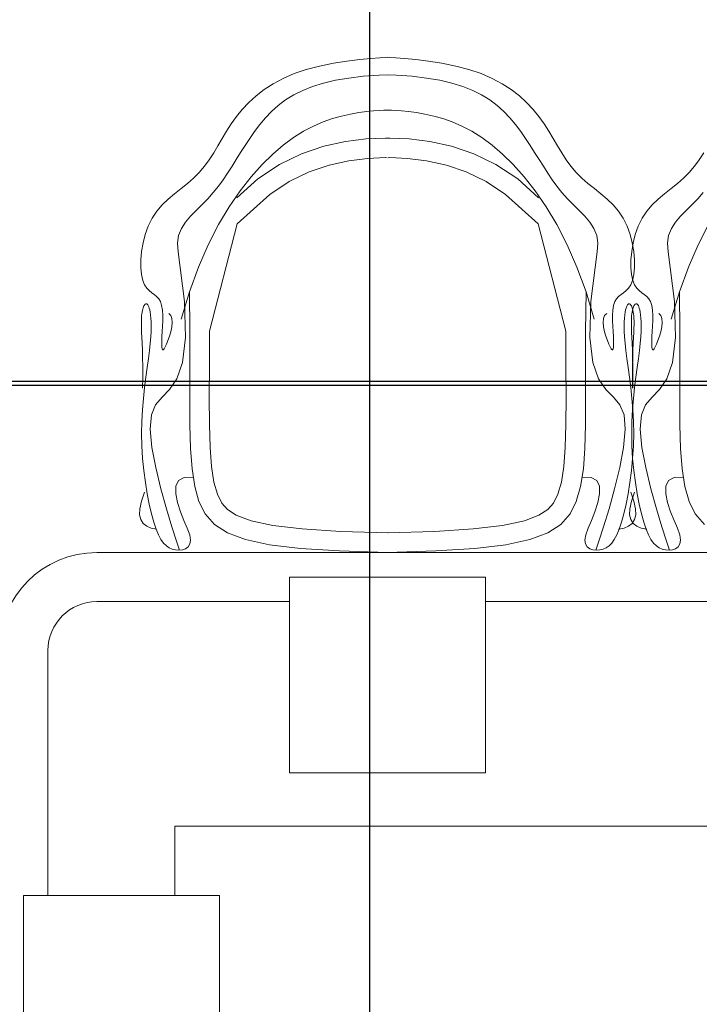
# Model space of a CAD drawing. Units: inches. Extents: x 1454 to 2136, y 626 to 1213.
# Tile 10 of 23: x 1592 to 1620, y 1101 to 1141. Entities that reach past the tile are written whole.
import ezdxf

# ---------------------------------------------------------------- set-up
doc = ezdxf.new("R2010")
doc.units = ezdxf.units.IN
doc.header["$MEASUREMENT"] = 0
for name, color, linetype, lineweight in [('A-ANNO-DIMS', 2, 'Continuous', 18), ('A-FURN-PATT', 252, 'Continuous', 13), ('conference', 41, 'Continuous', 18)]:
    doc.layers.add(name, color=color, linetype=linetype, lineweight=lineweight)
doc.styles.get("Standard").update_dxf_attribs({"font": 'arial.ttf'})
doc.dimstyles.get("Standard").update_dxf_attribs({"dimtxt": 4, "dimasz": 0.18, "dimexe": 0.18, "dimexo": 0.0625, "dimgap": 0.09, "dimtad": 0, "dimtih": 1, "dimtoh": 1, "dimdec": 0, "dimrnd": 6, "dimzin": 0, "dimdsep": 46, "dimlunit": 3, "dimtxsty": 'Standard', "dimcen": 0.09, "dimadec": 0, "dimazin": 0, "dimtfac": 1, "dimtdec": 0, "dimtofl": 0, "dimtmove": 0, "dimatfit": 3, "dimfxl": 1, "dimtolj": 1, "dimtzin": 0, "dimarcsym": 0})

# ---------------------------------------------------------------- blocks, each defined once
blk = doc.blocks.new('ОГ52_на12персон_стол2800х900')
for p, q in [((-1020.6, 783.7), (-1011.5, 784.5)), ((-1011.5, 784.5), (-1005.6, 784.9)), ((-1005.6, 784.9), (-1003.4, 785)), ((-1001.2, 784.9), (-1003.4, 785)), ((-995.2, 784.5), (-1001.2, 784.9)), ((-986.2, 783.7), (-995.2, 784.5)), ((-1086.4, 772.5), (-1072.8, 776)), ((-1072.8, 776), (-1058.8, 778.8)), ((-1058.8, 778.8), (-1044.9, 780.9)), ((-1044.9, 780.9), (-1031.9, 782.6)), ((-1031.9, 782.6), (-1020.6, 783.7)), ((-974.8, 782.6), (-986.2, 783.7)), ((-961.8, 780.9), (-974.8, 782.6)), ((-948, 778.8), (-961.8, 780.9)), ((-933.9, 776), (-948, 778.8)), ((-920.4, 772.5), (-933.9, 776)), ((-1110.1, 763.4), (-1098.8, 768.3)), ((-1098.8, 768.3), (-1086.4, 772.5)), ((-1043.1, 763.8), (-1028.3, 765.6)), ((-1028.3, 765.6), (-1012, 766.8)), ((-1012, 766.8), (-1003.4, 767.1)), ((-994.8, 766.8), (-1003.4, 767.1)), ((-978.4, 765.6), (-994.8, 766.8)), ((-963.6, 763.8), (-978.4, 765.6)), ((-907.9, 768.3), (-920.4, 772.5)), ((-896.6, 763.4), (-907.9, 768.3)), ((-1129.5, 752), (-1120.3, 758)), ((-1120.3, 758), (-1110.1, 763.4)), ((-1090.1, 751.2), (-1080, 755.2)), ((-1080, 755.2), (-1068.9, 758.7)), ((-1068.9, 758.7), (-1056.7, 761.5)), ((-1056.7, 761.5), (-1043.1, 763.8)), ((-950.1, 761.5), (-963.6, 763.8)), ((-937.8, 758.7), (-950.1, 761.5)), ((-926.7, 755.2), (-937.8, 758.7)), ((-916.6, 751.2), (-926.7, 755.2)), ((-886.5, 758), (-896.6, 763.4)), ((-877.3, 752), (-886.5, 758)), ((-1145.1, 738.8), (-1137.7, 745.6)), ((-1137.7, 745.6), (-1129.5, 752)), ((-1107.5, 741.4), (-1099.2, 746.6)), ((-1099.2, 746.6), (-1090.1, 751.2)), ((-907.5, 746.6), (-916.6, 751.2)), ((-899.2, 741.4), (-907.5, 746.6)), ((-869, 745.6), (-877.3, 752)), ((-861.6, 738.8), (-869, 745.6)), ((-1151.7, 731.7), (-1145.1, 738.8)), ((-1121.9, 729.6), (-1115, 735.7)), ((-1115, 735.7), (-1107.5, 741.4)), ((-891.7, 735.7), (-899.2, 741.4)), ((-884.9, 729.6), (-891.7, 735.7)), ((-855, 731.7), (-861.6, 738.8)), ((-1162.9, 716.9), (-1157.6, 724.4)), ((-1157.6, 724.4), (-1151.7, 731.7)), ((-1128.1, 723.1), (-1121.9, 729.6)), ((-1059.7, 722.3), (-1050.4, 724.9)), ((-1050.4, 724.9), (-1041.3, 727)), ((-1041.3, 727), (-1032.7, 728.5)), ((-1032.7, 728.5), (-1024.7, 729.6)), ((-1024.7, 729.6), (-1017.7, 730.4)), ((-1017.7, 730.4), (-1011.8, 730.8)), ((-1011.8, 730.8), (-1007.3, 731)), ((-1007.3, 731), (-1004.4, 731.1)), ((-1004.4, 731.1), (-1003.4, 731.1)), ((-1002.3, 731.1), (-1003.4, 731.1)), ((-999.4, 731), (-1002.3, 731.1)), ((-994.9, 730.8), (-999.4, 731)), ((-989.1, 730.4), (-994.9, 730.8)), ((-982, 729.6), (-989.1, 730.4)), ((-974.1, 728.5), (-982, 729.6)), ((-965.4, 727), (-974.1, 728.5)), ((-956.3, 724.9), (-965.4, 727)), ((-947, 722.3), (-956.3, 724.9)), ((-878.6, 723.1), (-884.9, 729.6)), ((-849.1, 724.4), (-855, 731.7)), ((-843.8, 716.9), (-849.1, 724.4)), ((-1167.7, 709.4), (-1162.9, 716.9)), ((-1139.2, 709.3), (-1133.9, 716.3)), ((-1133.9, 716.3), (-1128.1, 723.1)), ((-1089.1, 709.4), (-1079.1, 714.7)), ((-1079.1, 714.7), (-1069.3, 718.9)), ((-1069.3, 718.9), (-1059.7, 722.3)), ((-937.4, 718.9), (-947, 722.3)), ((-927.6, 714.7), (-937.4, 718.9)), ((-917.6, 709.4), (-927.6, 714.7)), ((-872.9, 716.3), (-878.6, 723.1)), ((-867.6, 709.3), (-872.9, 716.3)), ((-839, 709.4), (-843.8, 716.9)), ((-1172.2, 701.9), (-1167.7, 709.4)), ((-1144.1, 702.2), (-1139.2, 709.3)), ((-1099.4, 703), (-1089.1, 709.4)), ((-907.4, 703), (-917.6, 709.4)), ((-862.6, 702.2), (-867.6, 709.3)), ((-834.5, 701.9), (-839, 709.4)), ((-1180.9, 687.3), (-1176.6, 694.5)), ((-1176.6, 694.5), (-1172.2, 701.9)), ((-1153.4, 687.9), (-1148.8, 695)), ((-1148.8, 695), (-1144.1, 702.2)), ((-1120.6, 686.1), (-1109.9, 695.3)), ((-1109.9, 695.3), (-1099.4, 703)), ((-1091.2, 686.5), (-1068.6, 694.2)), ((-1068.6, 694.2), (-1046.5, 699)), ((-1046.5, 699), (-1025.4, 701.6)), ((-1025.4, 701.6), (-1005.7, 702.5)), ((-1005.7, 702.5), (-1003.4, 702.4)), ((-1001, 702.5), (-1003.4, 702.4)), ((-981.3, 701.6), (-1001, 702.5)), ((-960.2, 699), (-981.3, 701.6)), ((-938.1, 694.2), (-960.2, 699)), ((-915.6, 686.5), (-938.1, 694.2)), ((-896.9, 695.3), (-907.4, 703)), ((-886.2, 686.1), (-896.9, 695.3)), ((-857.9, 695), (-862.6, 702.2)), ((-853.4, 687.9), (-857.9, 695)), ((-830.2, 694.5), (-834.5, 701.9)), ((-825.8, 687.3), (-830.2, 694.5)), ((-1185.4, 680.3), (-1180.9, 687.3)), ((-1157.8, 680.7), (-1153.4, 687.9)), ((-1131.5, 675.4), (-1120.6, 686.1)), ((-1113.8, 675.6), (-1091.2, 686.5)), ((-893, 675.6), (-915.6, 686.5)), ((-875.2, 675.4), (-886.2, 686.1)), ((-848.9, 680.7), (-853.4, 687.9)), ((-821.3, 680.3), (-825.8, 687.3)), ((-685.4, 680.3), (-680.9, 687.3)), ((-1195.6, 667.5), (-1190.3, 673.7)), ((-1190.3, 673.7), (-1185.4, 680.3)), ((-1166.7, 666.7), (-1162.2, 673.7)), ((-1162.2, 673.7), (-1157.8, 680.7)), ((-1142.7, 663), (-1131.5, 675.4)), ((-1136, 660.8), (-1113.8, 675.6)), ((-1083.6, 668), (-1063.2, 674.9)), ((-1063.2, 674.9), (-1043.1, 679.3)), ((-1043.1, 679.3), (-1023.8, 681.7)), ((-1023.8, 681.7), (-1005.5, 682.5)), ((-1005.5, 682.5), (-1003.8, 682.4)), ((-1001.3, 682.5), (-1003, 682.4)), ((-983, 681.7), (-1001.3, 682.5)), ((-963.6, 679.3), (-983, 681.7)), ((-943.5, 674.9), (-963.6, 679.3)), ((-923.2, 668), (-943.5, 674.9)), ((-870.7, 660.8), (-893, 675.6)), ((-864, 663), (-875.2, 675.4)), ((-844.5, 673.7), (-848.9, 680.7)), ((-840.1, 666.7), (-844.5, 673.7)), ((-816.5, 673.7), (-821.3, 680.3)), ((-811.2, 667.5), (-816.5, 673.7)), ((-695.6, 667.5), (-690.3, 673.7)), ((-690.3, 673.7), (-685.4, 680.3)), ((-1201.4, 661.7), (-1195.6, 667.5)), ((-1171.3, 659.9), (-1166.7, 666.7)), ((-1103.8, 658.2), (-1083.6, 668)), ((-902.9, 658.2), (-923.2, 668)), ((-835.5, 659.9), (-840.1, 666.7)), ((-805.3, 661.7), (-811.2, 667.5)), ((-701.4, 661.7), (-695.6, 667.5)), ((-1214.2, 650.9), (-1207.7, 656.2)), ((-1207.7, 656.2), (-1201.4, 661.7)), ((-1176.1, 653.3), (-1171.3, 659.9)), ((-1157.3, 641.6), (-1136, 660.8)), ((-1154, 648.7), (-1142.7, 663)), ((-1123.7, 644.9), (-1103.8, 658.2)), ((-883, 644.9), (-902.9, 658.2)), ((-849.4, 641.6), (-870.7, 660.8)), ((-852.8, 648.7), (-864, 663)), ((-830.6, 653.3), (-835.5, 659.9)), ((-799, 656.2), (-805.3, 661.7)), ((-792.5, 650.9), (-799, 656.2)), ((-714.2, 650.9), (-707.7, 656.2)), ((-707.7, 656.2), (-701.4, 661.7)), ((-1227.3, 640.1), (-1220.8, 645.6)), ((-1220.8, 645.6), (-1214.2, 650.9)), ((-1186.8, 640.6), (-1181.3, 646.8)), ((-1181.3, 646.8), (-1176.1, 653.3)), ((-1165.2, 632.4), (-1154, 648.7)), ((-1157, 615), (-1123.7, 644.9)), ((-849.8, 615), (-883, 644.9)), ((-841.6, 632.4), (-852.8, 648.7)), ((-825.5, 646.8), (-830.6, 653.3)), ((-820, 640.6), (-825.5, 646.8)), ((-785.9, 645.6), (-792.5, 650.9)), ((-779.5, 640.1), (-785.9, 645.6)), ((-727.3, 640.1), (-720.8, 645.6)), ((-720.8, 645.6), (-714.2, 650.9)), ((-686.8, 640.6), (-681.3, 646.8)), ((-1238.9, 627.7), (-1233.4, 634.2)), ((-1233.4, 634.2), (-1227.3, 640.1)), ((-1198.7, 628.7), (-1192.7, 634.6)), ((-1192.7, 634.6), (-1186.8, 640.6)), ((-814.1, 634.6), (-820, 640.6)), ((-808, 628.7), (-814.1, 634.6)), ((-773.4, 634.2), (-779.5, 640.1)), ((-767.8, 627.7), (-773.4, 634.2)), ((-738.9, 627.7), (-733.4, 634.2)), ((-733.4, 634.2), (-727.3, 640.1)), ((-698.7, 628.7), (-692.7, 634.6)), ((-692.7, 634.6), (-686.8, 640.6)), ((-1243.7, 620.6), (-1238.9, 627.7)), ((-1204.5, 622.8), (-1198.7, 628.7)), ((-1176.1, 614.1), (-1165.2, 632.4)), ((-830.7, 614.1), (-841.6, 632.4)), ((-802.3, 622.8), (-808, 628.7)), ((-763, 620.6), (-767.8, 627.7)), ((-743.7, 620.6), (-738.9, 627.7)), ((-704.5, 622.8), (-698.7, 628.7)), ((-1247.7, 612.7), (-1243.7, 620.6)), ((-1213.8, 610.1), (-1209.6, 616.6)), ((-1209.6, 616.6), (-1204.5, 622.8)), ((-1186.6, 593.6), (-1176.1, 614.1)), ((-1157, 615), (-1185.3, 505.2)), ((-849.8, 615), (-821.5, 505.2)), ((-820.1, 593.6), (-830.7, 614.1)), ((-797.1, 616.6), (-802.3, 622.8)), ((-792.9, 610.1), (-797.1, 616.6)), ((-759.1, 612.7), (-763, 620.6)), ((-747.7, 612.7), (-743.7, 620.6)), ((-713.8, 610.1), (-709.6, 616.6)), ((-709.6, 616.6), (-704.5, 622.8)), ((-686.6, 593.6), (-676.1, 614.1)), ((-1253, 595.4), (-1250.7, 604.2)), ((-1250.7, 604.2), (-1247.7, 612.7)), ((-1216.7, 603), (-1213.8, 610.1)), ((-790, 603), (-792.9, 610.1)), ((-756, 604.2), (-759.1, 612.7)), ((-753.8, 595.4), (-756, 604.2)), ((-753, 595.4), (-750.7, 604.2)), ((-750.7, 604.2), (-747.7, 612.7)), ((-716.7, 603), (-713.8, 610.1)), ((-1254.4, 586.6), (-1253, 595.4)), ((-1217.9, 595.2), (-1216.7, 603)), ((-1217.1, 586.5), (-1217.9, 595.2)), ((-1196.5, 570.7), (-1186.6, 593.6)), ((-810.2, 570.7), (-820.1, 593.6)), ((-788.8, 595.2), (-790, 603)), ((-789.6, 586.5), (-788.8, 595.2)), ((-754.4, 586.6), (-753, 595.4)), ((-752.3, 586.6), (-753.8, 595.4)), ((-717.9, 595.2), (-716.7, 603)), ((-717.1, 586.5), (-717.9, 595.2)), ((-696.5, 570.7), (-686.6, 593.6)), ((-1255.1, 578.1), (-1254.4, 586.6)), ((-1217.1, 586.5), (-1210.8, 535.5)), ((-789.6, 586.5), (-796, 535.5)), ((-755.1, 578.1), (-754.4, 586.6)), ((-751.6, 578.1), (-752.3, 586.6)), ((-717.1, 586.5), (-710.8, 535.5)), ((-1255.1, 570.2), (-1255.1, 578.1)), ((-755.1, 570.2), (-755.1, 578.1)), ((-751.6, 570.2), (-751.6, 578.1)), ((-1254.5, 563.1), (-1255.1, 570.2)), ((-1253.2, 557.2), (-1254.5, 563.1)), ((-1205.7, 545.4), (-1196.5, 570.7)), ((-801, 545.4), (-810.2, 570.7)), ((-754.5, 563.1), (-755.1, 570.2)), ((-753.2, 557.2), (-754.5, 563.1)), ((-753.5, 557.2), (-752.3, 563.1)), ((-752.3, 563.1), (-751.6, 570.2)), ((-705.7, 545.4), (-696.5, 570.7)), ((-1251.4, 552.7), (-1253.2, 557.2)), ((-755.3, 552.7), (-753.5, 557.2)), ((-751.4, 552.7), (-753.2, 557.2)), ((-1249.2, 549.3), (-1251.4, 552.7)), ((-1246.7, 546.7), (-1249.2, 549.3)), ((-1244.1, 544.6), (-1246.7, 546.7)), ((-1241.5, 542.8), (-1244.1, 544.6)), ((-1214, 517.6), (-1205.7, 545.4)), ((-1205.7, 545.4), (-1205.3, 505.1)), ((-801, 545.4), (-801.5, 505.1)), ((-792.7, 517.6), (-801, 545.4)), ((-765.2, 542.8), (-762.6, 544.6)), ((-762.6, 544.6), (-760, 546.7)), ((-760, 546.7), (-757.5, 549.3)), ((-757.5, 549.3), (-755.3, 552.7)), ((-749.2, 549.3), (-751.4, 552.7)), ((-746.7, 546.7), (-749.2, 549.3)), ((-744.1, 544.6), (-746.7, 546.7)), ((-741.5, 542.8), (-744.1, 544.6)), ((-714, 517.6), (-705.7, 545.4)), ((-705.7, 545.4), (-705.3, 505.1)), ((-1250.7, 533), (-1251.2, 532.5)), ((-1250.2, 533.2), (-1250.7, 533)), ((-1249.7, 533.3), (-1250.2, 533.2)), ((-1249.2, 533.2), (-1249.7, 533.3)), ((-1248.7, 532.9), (-1249.2, 533.2)), ((-1248.1, 532.3), (-1248.7, 532.9)), ((-1239.1, 540.8), (-1241.5, 542.8)), ((-1236.9, 538.5), (-1239.1, 540.8)), ((-1235.2, 535.5), (-1236.9, 538.5)), ((-1234, 531.5), (-1235.2, 535.5)), ((-1210.8, 535.5), (-1209.7, 498.8)), ((-796, 535.5), (-797, 498.8)), ((-772.8, 531.5), (-771.6, 535.5)), ((-771.6, 535.5), (-769.8, 538.5)), ((-769.8, 538.5), (-767.7, 540.8)), ((-767.7, 540.8), (-765.2, 542.8)), ((-758.6, 532.3), (-758.1, 532.9)), ((-758.1, 532.9), (-757.6, 533.2)), ((-757.6, 533.2), (-757, 533.3)), ((-757, 533.3), (-756.5, 533.2)), ((-756.5, 533.2), (-756, 533)), ((-756, 533), (-755.6, 532.5)), ((-750.7, 533), (-751.2, 532.5)), ((-750.2, 533.2), (-750.7, 533)), ((-749.7, 533.3), (-750.2, 533.2)), ((-749.2, 533.2), (-749.7, 533.3)), ((-748.7, 532.9), (-749.2, 533.2)), ((-748.1, 532.3), (-748.7, 532.9)), ((-739.1, 540.8), (-741.5, 542.8)), ((-736.9, 538.5), (-739.1, 540.8)), ((-735.2, 535.5), (-736.9, 538.5)), ((-734, 531.5), (-735.2, 535.5)), ((-710.8, 535.5), (-709.7, 498.8)), ((-1254.2, 523.1), (-1254.5, 521)), ((-1254, 524.9), (-1254.2, 523.1)), ((-1253.6, 526.5), (-1254, 524.9)), ((-1253.3, 527.9), (-1253.6, 526.5)), ((-1252.9, 529.1), (-1253.3, 527.9)), ((-1252.5, 530.2), (-1252.9, 529.1)), ((-1252.1, 531.1), (-1252.5, 530.2)), ((-1251.6, 531.9), (-1252.1, 531.1)), ((-1251.2, 532.5), (-1251.6, 531.9)), ((-1247.6, 531.5), (-1248.1, 532.3)), ((-1247.1, 530.3), (-1247.6, 531.5)), ((-1246.6, 528.8), (-1247.1, 530.3)), ((-1246.2, 527), (-1246.6, 528.8)), ((-1245.7, 524.7), (-1246.2, 527)), ((-1245.3, 521.9), (-1245.7, 524.7)), ((-1233.3, 526.8), (-1234, 531.5)), ((-1232.9, 521.5), (-1233.3, 526.8)), ((-1226.8, 523.4), (-1224.6, 521.4)), ((-779.9, 523.4), (-782.1, 521.4)), ((-773.8, 521.5), (-773.5, 526.8)), ((-773.5, 526.8), (-772.8, 531.5)), ((-761.4, 521.9), (-761, 524.7)), ((-761, 524.7), (-760.6, 527)), ((-760.6, 527), (-760.1, 528.8)), ((-760.1, 528.8), (-759.6, 530.3)), ((-759.6, 530.3), (-759.1, 531.5)), ((-759.1, 531.5), (-758.6, 532.3)), ((-755.6, 532.5), (-755.1, 531.9)), ((-755.1, 531.9), (-754.7, 531.1)), ((-754.7, 531.1), (-754.2, 530.2)), ((-754.2, 523.1), (-754.5, 521)), ((-754.2, 530.2), (-753.8, 529.1)), ((-754, 524.9), (-754.2, 523.1)), ((-753.6, 526.5), (-754, 524.9)), ((-753.8, 529.1), (-753.5, 527.9)), ((-753.3, 527.9), (-753.6, 526.5)), ((-753.5, 527.9), (-753.1, 526.5)), ((-752.9, 529.1), (-753.3, 527.9)), ((-753.1, 526.5), (-752.8, 524.9)), ((-752.5, 530.2), (-752.9, 529.1)), ((-752.8, 524.9), (-752.5, 523.1)), ((-752.1, 531.1), (-752.5, 530.2)), ((-752.5, 523.1), (-752.3, 521)), ((-751.6, 531.9), (-752.1, 531.1)), ((-751.2, 532.5), (-751.6, 531.9)), ((-747.6, 531.5), (-748.1, 532.3)), ((-747.1, 530.3), (-747.6, 531.5)), ((-746.6, 528.8), (-747.1, 530.3)), ((-746.2, 527), (-746.6, 528.8)), ((-745.7, 524.7), (-746.2, 527)), ((-745.3, 521.9), (-745.7, 524.7)), ((-733.3, 526.8), (-734, 531.5)), ((-732.9, 521.5), (-733.3, 526.8)), ((-726.8, 523.4), (-724.6, 521.4)), ((-1254.6, 518.5), (-1254.7, 515.7)), ((-1254.7, 515.7), (-1254.7, 512.3)), ((-1254.5, 521), (-1254.6, 518.5)), ((-1245, 518.7), (-1245.3, 521.9)), ((-1244.8, 514.9), (-1245, 518.7)), ((-1244.7, 510.5), (-1244.8, 514.9)), ((-1233.1, 510.3), (-1232.9, 516)), ((-1232.9, 516), (-1232.9, 521.5)), ((-1224.6, 521.4), (-1223.5, 518.2)), ((-1223.3, 514.2), (-1223.7, 509.6)), ((-1223.5, 518.2), (-1223.3, 514.2)), ((-783.2, 518.2), (-783.5, 514.2)), ((-783.5, 514.2), (-783, 509.6)), ((-782.1, 521.4), (-783.2, 518.2)), ((-773.8, 516), (-773.8, 521.5)), ((-773.6, 510.3), (-773.8, 516)), ((-762, 510.5), (-761.9, 514.9)), ((-761.9, 514.9), (-761.7, 518.7)), ((-761.7, 518.7), (-761.4, 521.9)), ((-754.6, 518.5), (-754.7, 515.7)), ((-754.7, 515.7), (-754.7, 512.3)), ((-754.5, 521), (-754.6, 518.5)), ((-752.3, 521), (-752.1, 518.5)), ((-752.1, 518.5), (-752, 515.7)), ((-752, 515.7), (-752, 512.3)), ((-745, 518.7), (-745.3, 521.9)), ((-744.8, 514.9), (-745, 518.7)), ((-744.7, 510.5), (-744.8, 514.9)), ((-733.1, 510.3), (-732.9, 516)), ((-732.9, 516), (-732.9, 521.5)), ((-724.6, 521.4), (-723.5, 518.2)), ((-723.3, 514.2), (-723.7, 509.6)), ((-723.5, 518.2), (-723.3, 514.2)), ((-1254.7, 512.3), (-1254.6, 508.5)), ((-1254.6, 508.5), (-1254.5, 504)), ((-1254.5, 504), (-1254.2, 498.9)), ((-1245.1, 499.6), (-1244.8, 505.4)), ((-1244.8, 505.4), (-1244.7, 510.5)), ((-1233.7, 499.8), (-1233.4, 504.9)), ((-1233.4, 504.9), (-1233.1, 510.3)), ((-1224.7, 504.8), (-1226.1, 500.1)), ((-1223.7, 509.6), (-1224.7, 504.8)), ((-1205.3, 505.1), (-1205.3, 469.2)), ((-1185.3, 505.2), (-1185.3, 469.2)), ((-821.5, 505.2), (-821.5, 469.2)), ((-801.5, 505.1), (-801.5, 469.2)), ((-783, 509.6), (-782, 504.8)), ((-782, 504.8), (-780.7, 500.1)), ((-773.4, 504.9), (-773.6, 510.3)), ((-773.1, 499.8), (-773.4, 504.9)), ((-762, 505.4), (-762, 510.5)), ((-761.7, 499.6), (-762, 505.4)), ((-754.7, 512.3), (-754.6, 508.5)), ((-754.6, 508.5), (-754.5, 504)), ((-754.5, 504), (-754.2, 498.9)), ((-752.3, 504), (-752.5, 498.9)), ((-752.1, 508.5), (-752.3, 504)), ((-752, 512.3), (-752.1, 508.5)), ((-745.1, 499.6), (-744.8, 505.4)), ((-744.8, 505.4), (-744.7, 510.5)), ((-733.7, 499.8), (-733.4, 504.9)), ((-733.4, 504.9), (-733.1, 510.3)), ((-724.7, 504.8), (-726.1, 500.1)), ((-723.7, 509.6), (-724.7, 504.8)), ((-705.3, 505.1), (-705.3, 469.2)), ((-1254.2, 498.9), (-1253.9, 493)), ((-1253.9, 493), (-1253.7, 486.1)), ((-1246.4, 485.6), (-1245.6, 493.1)), ((-1245.6, 493.1), (-1245.1, 499.6)), ((-1233.9, 495.4), (-1233.7, 499.8)), ((-1233.9, 491.8), (-1233.9, 495.4)), ((-1227.6, 495.7), (-1229, 492)), ((-1226.1, 500.1), (-1227.6, 495.7)), ((-1209.7, 498.8), (-1212.8, 473.4)), ((-797, 498.8), (-794, 473.4)), ((-780.7, 500.1), (-779.2, 495.7)), ((-779.2, 495.7), (-777.7, 492)), ((-772.9, 495.4), (-773.1, 499.8)), ((-772.8, 491.8), (-772.9, 495.4)), ((-761.2, 493.1), (-761.7, 499.6)), ((-760.4, 485.6), (-761.2, 493.1)), ((-754.2, 498.9), (-753.9, 493)), ((-753.9, 493), (-753.7, 486.1)), ((-752.8, 493), (-753.1, 486.1)), ((-752.5, 498.9), (-752.8, 493)), ((-746.4, 485.6), (-745.6, 493.1)), ((-745.6, 493.1), (-745.1, 499.6)), ((-733.9, 495.4), (-733.7, 499.8)), ((-733.9, 491.8), (-733.9, 495.4)), ((-727.6, 495.7), (-729, 492)), ((-726.1, 500.1), (-727.6, 495.7)), ((-709.7, 498.8), (-712.8, 473.4)), ((-1253.7, 486.1), (-1253.4, 478.2)), ((-1247.4, 477.3), (-1246.4, 485.6)), ((-1233.8, 489.1), (-1233.9, 491.8)), ((-1233.5, 487.3), (-1233.8, 489.1)), ((-1233, 486.4), (-1233.5, 487.3)), ((-1232.3, 486.4), (-1233, 486.4)), ((-1231.4, 487.3), (-1232.3, 486.4)), ((-1230.3, 489.2), (-1231.4, 487.3)), ((-1229, 492), (-1230.3, 489.2)), ((-777.7, 492), (-776.4, 489.2)), ((-776.4, 489.2), (-775.3, 487.3)), ((-775.3, 487.3), (-774.4, 486.4)), ((-774.4, 486.4), (-773.8, 486.4)), ((-773.8, 486.4), (-773.3, 487.3)), ((-773.3, 487.3), (-772.9, 489.1)), ((-772.9, 489.1), (-772.8, 491.8)), ((-759.3, 477.3), (-760.4, 485.6)), ((-753.7, 486.1), (-753.4, 478.2)), ((-753.1, 486.1), (-753.3, 478.2)), ((-747.4, 477.3), (-746.4, 485.6)), ((-733.8, 489.1), (-733.9, 491.8)), ((-733.5, 487.3), (-733.8, 489.1)), ((-733, 486.4), (-733.5, 487.3)), ((-732.3, 486.4), (-733, 486.4)), ((-731.4, 487.3), (-732.3, 486.4)), ((-730.3, 489.2), (-731.4, 487.3)), ((-729, 492), (-730.3, 489.2)), ((-1253.4, 478.2), (-1253.3, 469.2)), ((-1248.7, 468.2), (-1247.4, 477.3)), ((-1212.8, 473.4), (-1218.6, 456.6)), ((-794, 473.4), (-788.1, 456.6)), ((-758, 468.2), (-759.3, 477.3)), ((-753.3, 478.2), (-753.4, 469.2)), ((-753.4, 478.2), (-753.3, 469.2)), ((-748.7, 468.2), (-747.4, 477.3)), ((-712.8, 473.4), (-718.6, 456.6)), ((-1253.3, 469.2), (-1253.3, 458.8)), ((-1250, 458.3), (-1248.7, 468.2)), ((-1205.3, 469.2), (-1205.4, 437.5)), ((-1185.3, 469.2), (-1185.4, 437.6)), ((-821.5, 469.2), (-821.4, 437.6)), ((-801.5, 469.2), (-801.4, 437.5)), ((-756.7, 458.3), (-758, 468.2)), ((-753.4, 469.2), (-753.5, 458.8)), ((-753.3, 469.2), (-753.3, 458.8)), ((-750, 458.3), (-748.7, 468.2)), ((-705.3, 469.2), (-705.4, 437.5)), ((-1253.3, 458.8), (-1253.4, 447.1)), ((-1251.4, 447.8), (-1250, 458.3)), ((-1218.6, 456.6), (-1226, 445.7)), ((-788.1, 456.6), (-780.7, 445.7)), ((-755.4, 447.8), (-756.7, 458.3)), ((-753.5, 458.8), (-753.3, 447.1)), ((-753.3, 458.8), (-753.4, 447.1)), ((-751.4, 447.8), (-750, 458.3)), ((-718.6, 456.6), (-726, 445.7)), ((-1252.6, 436.7), (-1251.4, 447.8)), ((-1226, 445.7), (-1233.6, 437.8)), ((-780.7, 445.7), (-773.1, 437.8)), ((-754.1, 436.7), (-755.4, 447.8)), ((-752.6, 436.7), (-751.4, 447.8)), ((-726, 445.7), (-733.6, 437.8)), ((-1253.6, 425.1), (-1252.6, 436.7)), ((-1233.6, 437.8), (-1240.2, 430.2)), ((-1205.4, 437.5), (-1205.3, 409.8)), ((-1185.4, 437.6), (-1185.3, 410.1)), ((-821.4, 437.6), (-821.5, 410.1)), ((-801.4, 437.5), (-801.5, 409.8)), ((-773.1, 437.8), (-766.5, 430.2)), ((-753.1, 425.1), (-754.1, 436.7)), ((-753.6, 425.1), (-752.6, 436.7)), ((-733.6, 437.8), (-740.2, 430.2)), ((-705.4, 437.5), (-705.3, 409.8)), ((-1254.2, 413.1), (-1253.6, 425.1)), ((-1240.2, 430.2), (-1244.5, 420)), ((-766.5, 430.2), (-762.2, 420)), ((-754.2, 413.1), (-753.6, 425.1)), ((-752.5, 413.1), (-753.1, 425.1)), ((-740.2, 430.2), (-744.5, 420)), ((-1254.4, 400.7), (-1254.2, 413.1)), ((-1244.5, 420), (-1245.6, 405.3)), ((-762.2, 420), (-761.1, 405.3)), ((-754.4, 400.7), (-754.2, 413.1)), ((-752.3, 400.7), (-752.5, 413.1)), ((-744.5, 420), (-745.6, 405.3)), ((-1245.6, 405.3), (-1243.9, 386.7)), ((-1205.3, 409.8), (-1204.6, 385.6)), ((-1185.3, 410.1), (-1184.6, 386.6)), ((-821.5, 410.1), (-822.1, 386.6)), ((-801.5, 409.8), (-802.2, 385.6)), ((-761.1, 405.3), (-762.8, 386.7)), ((-745.6, 405.3), (-743.9, 386.7)), ((-705.3, 409.8), (-704.6, 385.6)), ((-1254.1, 388.2), (-1254.4, 400.7)), ((-754.1, 388.2), (-754.4, 400.7)), ((-752.6, 388.2), (-752.3, 400.7)), ((-1253.4, 375.5), (-1254.1, 388.2)), ((-1243.9, 386.7), (-1240.1, 366)), ((-1204.6, 385.6), (-1203, 364.7)), ((-1184.6, 386.6), (-1183.1, 367)), ((-822.1, 386.6), (-823.6, 367)), ((-802.2, 385.6), (-803.7, 364.7)), ((-762.8, 386.7), (-766.6, 366)), ((-753.4, 375.5), (-754.1, 388.2)), ((-753.4, 375.5), (-752.6, 388.2)), ((-743.9, 386.7), (-740.1, 366)), ((-704.6, 385.6), (-703, 364.7)), ((-1252.1, 363), (-1253.4, 375.5)), ((-754.6, 363), (-753.4, 375.5)), ((-752.1, 363), (-753.4, 375.5)), ((-1250.6, 350.9), (-1252.1, 363)), ((-1240.1, 366), (-1235, 344.5)), ((-1203, 364.7), (-1200.2, 346.8)), ((-1183.1, 367), (-1180.6, 351.1)), ((-823.6, 367), (-826.1, 351.1)), ((-803.7, 364.7), (-806.5, 346.8)), ((-766.6, 366), (-771.8, 344.5)), ((-756.2, 350.9), (-754.6, 363)), ((-750.6, 350.9), (-752.1, 363)), ((-740.1, 366), (-735, 344.5)), ((-703, 364.7), (-700.2, 346.8)), ((-1219.4, 347.1), (-1216.8, 353)), ((-1216.8, 353), (-1211.1, 356.1)), ((-1211.1, 356.1), (-1201.6, 355.7)), ((-795.6, 356.1), (-805.1, 355.7)), ((-789.9, 353), (-795.6, 356.1)), ((-787.3, 347.1), (-789.9, 353)), ((-719.4, 347.1), (-716.8, 353)), ((-716.8, 353), (-711.1, 356.1)), ((-711.1, 356.1), (-701.6, 355.7)), ((-1248.7, 339.4), (-1250.6, 350.9)), ((-1235, 344.5), (-1229.2, 323.8)), ((-1219.5, 339.3), (-1219.4, 347.1)), ((-1200.2, 346.8), (-1195.9, 331.5)), ((-1180.6, 351.1), (-1177.1, 338.8)), ((-826.1, 351.1), (-829.6, 338.8)), ((-806.5, 346.8), (-810.9, 331.5)), ((-787.3, 339.3), (-787.3, 347.1)), ((-771.8, 344.5), (-777.5, 323.8)), ((-758, 339.4), (-756.2, 350.9)), ((-748.7, 339.4), (-750.6, 350.9)), ((-735, 344.5), (-729.2, 323.8)), ((-719.5, 339.3), (-719.4, 347.1)), ((-700.2, 346.8), (-695.9, 331.5)), ((-1254.7, 331.8), (-1256.3, 324.1)), ((-1251.4, 341), (-1254.7, 331.8)), ((-1246.6, 328.7), (-1248.7, 339.4)), ((-1217.7, 330.3), (-1219.5, 339.3)), ((-1177.1, 338.8), (-1172.7, 329.9)), ((-829.6, 338.8), (-834, 329.9)), ((-789.1, 330.3), (-787.3, 339.3)), ((-760.1, 328.7), (-758, 339.4)), ((-754.7, 331.8), (-756.3, 324.1)), ((-755.4, 341), (-752.1, 331.8)), ((-751.4, 341), (-754.7, 331.8)), ((-752.1, 331.8), (-750.4, 324.1)), ((-746.6, 328.7), (-748.7, 339.4)), ((-717.7, 330.3), (-719.5, 339.3)), ((-1256.3, 324.1), (-1256.5, 317.8)), ((-1244.4, 318.9), (-1246.6, 328.7)), ((-1229.2, 323.8), (-1223.6, 305.4)), ((-1214.7, 321), (-1217.7, 330.3)), ((-1195.9, 331.5), (-1189.5, 318.7)), ((-1172.7, 329.9), (-1166.9, 323.3)), ((-1166.9, 323.3), (-1157.8, 317.4)), ((-839.8, 323.3), (-849, 317.4)), ((-834, 329.9), (-839.8, 323.3)), ((-810.9, 331.5), (-817.3, 318.7)), ((-792, 321), (-789.1, 330.3)), ((-777.5, 323.8), (-783.1, 305.4)), ((-762.3, 318.9), (-760.1, 328.7)), ((-756.3, 324.1), (-756.5, 317.8)), ((-750.4, 324.1), (-750.2, 317.8)), ((-744.4, 318.9), (-746.6, 328.7)), ((-729.2, 323.8), (-723.6, 305.4)), ((-714.7, 321), (-717.7, 330.3)), ((-695.9, 331.5), (-689.5, 318.7)), ((-1256.5, 317.8), (-1255.3, 312.9)), ((-1255.3, 312.9), (-1252.8, 309)), ((-1242.1, 310.4), (-1244.4, 318.9)), ((-1211.2, 312), (-1214.7, 321)), ((-1207.8, 304.2), (-1211.2, 312)), ((-1189.5, 318.7), (-1180.2, 308)), ((-1157.8, 317.4), (-1142.8, 311.8)), ((-1142.8, 311.8), (-1120.7, 307)), ((-863.9, 311.8), (-886.1, 307)), ((-849, 317.4), (-863.9, 311.8)), ((-817.3, 318.7), (-826.6, 308)), ((-798.9, 304.2), (-795.5, 312)), ((-795.5, 312), (-792, 321)), ((-764.7, 310.4), (-762.3, 318.9)), ((-756.5, 317.8), (-755.3, 312.9)), ((-755.3, 312.9), (-752.8, 309)), ((-751.5, 312.9), (-754, 309)), ((-750.2, 317.8), (-751.5, 312.9)), ((-742.1, 310.4), (-744.4, 318.9)), ((-711.2, 312), (-714.7, 321)), ((-707.8, 304.2), (-711.2, 312)), ((-689.5, 318.7), (-680.2, 308)), ((-1252.8, 309), (-1249.2, 306.2)), ((-1249.2, 306.2), (-1244.6, 304.3)), ((-1244.6, 304.3), (-1239.1, 303.1)), ((-1239.7, 303.2), (-1242.1, 310.4)), ((-1237.2, 297.3), (-1239.7, 303.2)), ((-1223.6, 305.4), (-1218.9, 291)), ((-1207.8, 304.2), (-1205.4, 297.4)), ((-1180.2, 308), (-1166.8, 299.4)), ((-1120.7, 307), (-1090.5, 303.4)), ((-1090.5, 303.4), (-1051.5, 300.9)), ((-916.3, 303.4), (-955.2, 300.9)), ((-886.1, 307), (-916.3, 303.4)), ((-826.6, 308), (-839.9, 299.4)), ((-798.9, 304.2), (-801.3, 297.4)), ((-783.1, 305.4), (-787.8, 291)), ((-769.5, 297.3), (-767.1, 303.2)), ((-762.2, 304.3), (-767.7, 303.1)), ((-767.1, 303.2), (-764.7, 310.4)), ((-757.6, 306.2), (-762.2, 304.3)), ((-754, 309), (-757.6, 306.2)), ((-752.8, 309), (-749.2, 306.2)), ((-749.2, 306.2), (-744.6, 304.3)), ((-744.6, 304.3), (-739.1, 303.1)), ((-739.7, 303.2), (-742.1, 310.4)), ((-737.2, 297.3), (-739.7, 303.2)), ((-723.6, 305.4), (-718.9, 291)), ((-707.8, 304.2), (-705.4, 297.4)), ((-1234.7, 292.5), (-1237.2, 297.3)), ((-1232, 288.8), (-1234.7, 292.5)), ((-1205.4, 297.4), (-1204.6, 292.1)), ((-1204.6, 292.1), (-1205.3, 288.1)), ((-1166.8, 299.4), (-1148.5, 292.5)), ((-1148.5, 292.5), (-1124, 287.3)), ((-1051.5, 300.9), (-1002.7, 299.3)), ((-955.2, 300.9), (-1004, 299.3)), ((-858.3, 292.5), (-882.8, 287.3)), ((-839.9, 299.4), (-858.3, 292.5)), ((-801.3, 297.4), (-802.1, 292.1)), ((-802.1, 292.1), (-801.5, 288.1)), ((-774.7, 288.8), (-772.1, 292.5)), ((-772.1, 292.5), (-769.5, 297.3)), ((-734.7, 292.5), (-737.2, 297.3)), ((-732, 288.8), (-734.7, 292.5)), ((-705.4, 297.4), (-704.6, 292.1)), ((-704.6, 292.1), (-705.3, 288.1)), ((-1229.2, 286.1), (-1232, 288.8)), ((-1226.3, 284.1), (-1229.2, 286.1)), ((-1223.2, 282.8), (-1226.3, 284.1)), ((-1219.8, 282.1), (-1223.2, 282.8)), ((-1216.3, 281.8), (-1219.8, 282.1)), ((-1218.9, 291), (-1215.9, 281.9)), ((-1212.8, 282.2), (-1216.3, 281.8)), ((-1209.6, 283.2), (-1212.8, 282.2)), ((-1207, 285.1), (-1209.6, 283.2)), ((-1205.3, 288.1), (-1207, 285.1)), ((-1124, 287.3), (-1092.3, 283.5)), ((-1092.3, 283.5), (-1052.5, 280.9)), ((-914.4, 283.5), (-954.3, 280.9)), ((-882.8, 287.3), (-914.4, 283.5)), ((-801.5, 288.1), (-799.7, 285.1)), ((-799.7, 285.1), (-797.1, 283.2)), ((-797.1, 283.2), (-793.9, 282.2)), ((-793.9, 282.2), (-790.4, 281.8)), ((-787.8, 291), (-790.9, 281.9)), ((-790.4, 281.8), (-786.9, 282.1)), ((-786.9, 282.1), (-783.6, 282.8)), ((-783.6, 282.8), (-780.4, 284.1)), ((-780.4, 284.1), (-777.5, 286.1)), ((-777.5, 286.1), (-774.7, 288.8)), ((-729.2, 286.1), (-732, 288.8)), ((-726.3, 284.1), (-729.2, 286.1)), ((-723.2, 282.8), (-726.3, 284.1)), ((-719.8, 282.1), (-723.2, 282.8)), ((-716.3, 281.8), (-719.8, 282.1)), ((-718.9, 291), (-715.9, 281.9)), ((-712.8, 282.2), (-716.3, 281.8)), ((-709.6, 283.2), (-712.8, 282.2)), ((-707, 285.1), (-709.6, 283.2)), ((-705.3, 288.1), (-707, 285.1)), ((-1300, 279.3), (1300, 279.3)), ((-1052.5, 280.9), (-1003.4, 279.3)), ((-954.3, 280.9), (-1003.4, 279.3)), ((-1103.4, 54.3), (-1103.4, 254.3)), ((-1103.4, 254.3), (-903.4, 254.3)), ((-903.4, 254.3), (-903.4, 54.3)), ((-1103.4, 229.3), (-1300, 229.3)), ((-603.4, 229.3), (-903.4, 229.3)), ((-1350, 179.3), (-1350, -70.7)), ((-903.4, 54.3), (-1103.4, 54.3)), ((1220.7, 0), (-1220.7, 0)), ((-1220.7, -70.7), (-1220.7, 0)), ((-1175, -70.7), (-1375, -70.7)), ((-1375, -70.7), (-1375, -270.7)), ((-1175, -270.7), (-1175, -70.7))]:
    blk.add_line(p, q)
for radius in [100, 50]:
    blk.add_arc((-1300, 179.3), radius, 90, 180)
blk = doc.blocks.new('*D23')
at = {"layer": 'A-ANNO-DIMS', "color": 0, "lineweight": -2, "transparency": 16777216}
for p, q in [((1571.674, 1139.532), (1571.674, 1162.157)), ((1721.725, 1139.532), (1721.725, 1162.157)), ((1571.854, 1161.977), (1615.675, 1161.977)), ((1721.545, 1161.977), (1677.724, 1161.977))]:
    blk.add_line(p, q, dxfattribs=at)
at = {"layer": 'A-ANNO-DIMS', "color": 0, "transparency": 16777216}
for points in [[(1571.854, 1162.007), (1571.854, 1161.947), (1571.674, 1161.977)], [(1721.545, 1162.007), (1721.545, 1161.947), (1721.725, 1161.977)]]:
    blk.add_solid(points, dxfattribs=at)
at = {"layer": 'Defpoints', "color": 0, "transparency": 16777216}
for p in [(1721.725, 1161.977), (1571.674, 1139.469), (1721.725, 1139.469)]:
    blk.add_point(p, dxfattribs=at)
at = {"layer": 'A-ANNO-DIMS', "color": 0, "transparency": 16777216, "insert": (1646.7, 1161.977), "char_height": 4, "attachment_point": 5}
blk.add_mtext('\\A1;CONFERENCE SET 150', dxfattribs=at)
blk = doc.blocks.new('*D33')
at = {"layer": 'A-ANNO-DIMS', "color": 0, "lineweight": -2, "transparency": 16777216}
for p, q in [((2032.494, 1126.282), (1462.374, 1126.282)), ((1462.554, 1126.102), (1462.554, 1056.381)), ((1462.554, 982.462), (1462.554, 1052.184)), ((2032.494, 982.282), (1462.374, 982.282))]:
    blk.add_line(p, q, dxfattribs=at)
at = {"layer": 'A-ANNO-DIMS', "color": 0, "transparency": 16777216}
for points in [[(1462.524, 1126.102), (1462.584, 1126.102), (1462.554, 1126.282)], [(1462.524, 982.462), (1462.584, 982.462), (1462.554, 982.282)]]:
    blk.add_solid(points, dxfattribs=at)
at = {"layer": 'Defpoints', "color": 0, "transparency": 16777216}
for p in [(1462.554, 1126.282), (2032.556, 1126.282), (2032.556, 982.282)]:
    blk.add_point(p, dxfattribs=at)
at = {"layer": 'A-ANNO-DIMS', "color": 0, "transparency": 16777216, "insert": (1462.554, 1054.282), "char_height": 4, "attachment_point": 5}
blk.add_mtext('\\A1;144', dxfattribs=at)
blk = doc.blocks.new('*D40')
at = {"layer": 'A-ANNO-DIMS', "color": 0, "lineweight": -2, "transparency": 16777216}
for p, q in [((1501.556, 877.345), (1501.556, 1210.464)), ((1501.736, 1210.284), (1569.244, 1210.284)), ((1645.376, 1210.284), (1577.869, 1210.284)), ((1645.556, 877.345), (1645.556, 1210.464))]:
    blk.add_line(p, q, dxfattribs=at)
at = {"layer": 'A-ANNO-DIMS', "color": 0, "transparency": 16777216}
for points in [[(1501.736, 1210.314), (1501.736, 1210.254), (1501.556, 1210.284)], [(1645.376, 1210.314), (1645.376, 1210.254), (1645.556, 1210.284)]]:
    blk.add_solid(points, dxfattribs=at)
at = {"layer": 'Defpoints', "color": 0, "transparency": 16777216}
for p in [(1645.556, 1210.284), (1501.556, 877.282), (1645.556, 877.282)]:
    blk.add_point(p, dxfattribs=at)
at = {"layer": 'A-ANNO-DIMS', "color": 0, "transparency": 16777216, "insert": (1573.556, 1210.284), "char_height": 4, "attachment_point": 5}
blk.add_mtext('\\A1;144', dxfattribs=at)
blk = doc.blocks.new('*D54')
at = {"layer": 'A-ANNO-DIMS', "color": 0, "lineweight": -2, "transparency": 16777216}
for p, q in [((1879.494, 1126.282), (1462.374, 1126.282)), ((1462.554, 1126.102), (1462.554, 1078.915)), ((1462.554, 1027.462), (1462.554, 1074.65)), ((1879.494, 1027.282), (1462.374, 1027.282))]:
    blk.add_line(p, q, dxfattribs=at)
at = {"layer": 'A-ANNO-DIMS', "color": 0, "transparency": 16777216}
for points in [[(1462.524, 1126.102), (1462.584, 1126.102), (1462.554, 1126.282)], [(1462.524, 1027.462), (1462.584, 1027.462), (1462.554, 1027.282)]]:
    blk.add_solid(points, dxfattribs=at)
at = {"layer": 'Defpoints', "color": 0, "transparency": 16777216}
for p in [(1879.556, 1126.282), (1462.554, 1027.282), (1879.556, 1027.282)]:
    blk.add_point(p, dxfattribs=at)
at = {"layer": 'A-ANNO-DIMS', "color": 0, "transparency": 16777216, "insert": (1462.554, 1076.782), "char_height": 4, "attachment_point": 5}
blk.add_mtext('\\A1;99', dxfattribs=at)
blk = doc.blocks.new('*D67')
at = {"layer": 'A-ANNO-DIMS', "color": 0, "lineweight": -2, "transparency": 16777216}
for p, q in [((1606.484, 1018.345), (1606.484, 1210.464)), ((1606.664, 1210.284), (1610.595, 1210.284)), ((1624.703, 1210.284), (1620.773, 1210.284)), ((1624.883, 1018.329), (1624.883, 1210.464))]:
    blk.add_line(p, q, dxfattribs=at)
at = {"layer": 'A-ANNO-DIMS', "color": 0, "transparency": 16777216}
for points in [[(1606.664, 1210.314), (1606.664, 1210.254), (1606.484, 1210.284)], [(1624.703, 1210.314), (1624.703, 1210.254), (1624.883, 1210.284)]]:
    blk.add_solid(points, dxfattribs=at)
at = {"layer": 'Defpoints', "color": 0, "transparency": 16777216}
for p in [(1624.883, 1210.284), (1606.484, 1018.282), (1624.883, 1018.267)]:
    blk.add_point(p, dxfattribs=at)
at = {"layer": 'A-ANNO-DIMS', "color": 0, "transparency": 16777216, "insert": (1615.684, 1210.284), "char_height": 4, "attachment_point": 5}
blk.add_mtext('\\A1;18.4', dxfattribs=at)
blk = doc.blocks.new('*D73')
at = {"layer": 'A-ANNO-DIMS', "color": 0, "lineweight": -2, "transparency": 16777216}
for p, q in [((1985.096, 1126.439), (1462.374, 1126.439)), ((1462.554, 1126.259), (1462.554, 1113.178)), ((1462.554, 1095.83), (1462.554, 1108.911)), ((1966.644, 1095.65), (1462.374, 1095.65))]:
    blk.add_line(p, q, dxfattribs=at)
at = {"layer": 'A-ANNO-DIMS', "color": 0, "transparency": 16777216}
for points in [[(1462.524, 1126.259), (1462.584, 1126.259), (1462.554, 1126.439)], [(1462.524, 1095.83), (1462.584, 1095.83), (1462.554, 1095.65)]]:
    blk.add_solid(points, dxfattribs=at)
at = {"layer": 'Defpoints', "color": 0, "transparency": 16777216}
for p in [(1985.158, 1126.439), (1462.554, 1095.65), (1966.707, 1095.65)]:
    blk.add_point(p, dxfattribs=at)
at = {"layer": 'A-ANNO-DIMS', "color": 0, "transparency": 16777216, "insert": (1462.554, 1111.044), "char_height": 4, "attachment_point": 5}
blk.add_mtext('\\A1;30.79', dxfattribs=at)

msp = doc.modelspace()

# ---------------------------------------------------------------- hatches: boundary and pattern name
at = {"layer": 'A-FURN-PATT'}
h = msp.add_hatch(dxfattribs=at)
h.set_pattern_fill('ESCHER', color=256)
h.paths.add_polyline_path([(1511.3761, 923.7174, 1), (1525.379, 923.7174, 1)])
h.paths.add_polyline_path([(1525.379, 816.0542, 1), (1511.3761, 816.0542, 1)])
h.paths.add_polyline_path([(1525.379, 712.7345, 1), (1511.3761, 712.7345, 1)])
h.paths.add_polyline_path([(2070.5057, 794.3402, 1), (2056.5027, 794.3402, 1)])
h.paths.add_polyline_path([(2005.868, 1014.5578, 1), (1991.8651, 1014.5578, 1)])
h.paths.add_polyline_path([(1994.0647, 1066.7584, 1), (2008.0677, 1066.7584, 1)])
h.paths.add_polyline_path([(1919.5492, 1065.3848, 1), (1933.5521, 1065.3848, 1)])
h.paths.add_polyline_path([(1936.8517, 1013.7336, 1), (1922.8488, 1013.7336, 1)])
h.paths.add_polyline_path([(1824.6062, 1109.1557, 1), (1838.6091, 1109.1557, 1)])

# ---------------------------------------------------------------- block references
at = {"layer": 'conference', "xscale": 0.0393700787401575, "yscale": 0.0393700787401575, "zscale": 0.0393700787401575}
msp.add_blockref('ОГ52_на12персон_стол2800х900', (1646.6996, 1108.5647), dxfattribs=at)

# ---------------------------------------------------------------- dimensions: what is measured, and where the dimension line sits
at = {"layer": 'A-ANNO-DIMS'}
for base, p1, p2, override, picture, middle in [((1645.5563, 1210.2845), (1501.5563, 877.2825), (1645.5563, 877.2825), {"dimdec": 0, "dimlfac": 1, "dimrnd": 0, "dimzin": 0, "dimdsep": 46, "dimlunit": 2}, '*D40', (1573.5563, 1210.2845)), ((1624.8835, 1210.2845), (1606.4844, 1018.2825), (1624.8835, 1018.2667), {"dimdec": 1, "dimlfac": 1, "dimrnd": 0, "dimzin": 0, "dimdsep": 46, "dimlunit": 2}, '*D67', (1615.6839, 1210.2845))]:
    dim = msp.add_linear_dim(base=base, p1=p1, p2=p2, dimstyle='Standard', override=override, dxfattribs=at)
    dim.commit()
    dim.dimension.update_dxf_attribs({"geometry": picture, "text_midpoint": middle})
dim = msp.add_linear_dim(base=(1721.7253, 1161.9768), p1=(1571.674, 1139.4691), p2=(1721.7253, 1139.4691), text='CONFERENCE SET <>', dimstyle='Standard', override={"dimdec": 0, "dimlfac": 1, "dimrnd": 0, "dimzin": 0, "dimdsep": 46, "dimlunit": 2}, dxfattribs=at)
dim.commit()
dim.dimension.update_dxf_attribs({"geometry": '*D23', "text_midpoint": (1646.6996, 1161.9768)})
for base, p1, p2, override, picture, middle in [((1462.5543, 1095.6495), (1985.1581, 1126.439), (1966.7068, 1095.6495), {"dimdec": 2, "dimlfac": 1, "dimrnd": 0, "dimzin": 0, "dimdsep": 46, "dimlunit": 2}, '*D73', (1462.5543, 1111.0443)), ((1462.5543, 1126.2825), (2032.5563, 982.2825), (2032.5563, 1126.2825), {"dimdec": 0, "dimlfac": 1, "dimrnd": 0, "dimzin": 0, "dimdsep": 46, "dimlunit": 2}, '*D33', (1462.5543, 1054.2825)), ((1462.5543, 1027.2825), (1879.5563, 1126.2825), (1879.5563, 1027.2825), {"dimdec": 0, "dimlfac": 1, "dimrnd": 0, "dimzin": 0, "dimdsep": 46, "dimlunit": 2}, '*D54', (1462.5543, 1076.7825))]:
    dim = msp.add_linear_dim(base=base, p1=p1, p2=p2, angle=90, dimstyle='Standard', override=override, dxfattribs=at)
    dim.commit()
    dim.dimension.update_dxf_attribs({"geometry": picture, "text_midpoint": middle})

doc.saveas('drawing.dxf')
